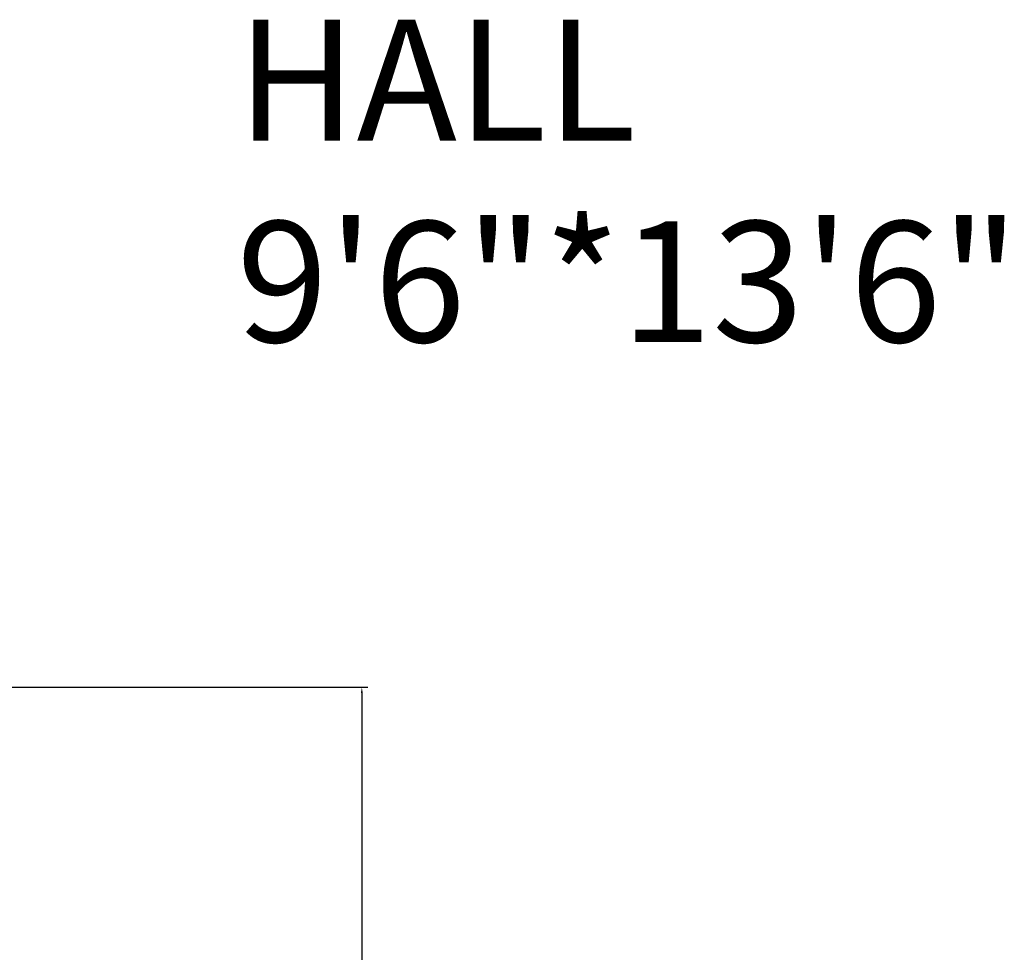
# Model space of a CAD drawing. Units: inches. Extents: x 1998 to 2588, y 1139 to 1977.
# Tile 55 of 134: x 2257 to 2287, y 1663 to 1692. Entities that reach past the tile are written whole.
import ezdxf

# ---------------------------------------------------------------- set-up
doc = ezdxf.new("R2010")
doc.units = ezdxf.units.IN
doc.layers.add('A-ANNO-DIMS', color=2, linetype='Continuous', lineweight=18)
doc.layers.add('A-AREA-IDEN', color=7, linetype='Continuous', lineweight=18)
doc.styles.get("Standard").update_dxf_attribs({"font": 'arial.ttf'})
doc.dimstyles.get("Standard").update_dxf_attribs({"dimtxt": 0.18, "dimasz": 0.18, "dimexe": 0.18, "dimexo": 0.0625, "dimgap": 0.09, "dimtad": 0, "dimtih": 1, "dimtoh": 1, "dimdec": 4, "dimzin": 0, "dimdsep": 46, "dimtxsty": 'Standard', "dimcen": 0.09, "dimadec": 0, "dimazin": 0, "dimtfac": 1, "dimtdec": 4, "dimtofl": 0, "dimtmove": 0, "dimatfit": 3, "dimfxl": 1, "dimtolj": 1, "dimtzin": 0, "dimarcsym": 0})

# ---------------------------------------------------------------- blocks, each defined once
blk = doc.blocks.new('*D11')
at = {"layer": 'A-ANNO-DIMS', "color": 0, "lineweight": -2, "transparency": 16777216}
for p, q in [((2256.378, 1671.356), (2267.646, 1671.356)), ((2267.466, 1671.176), (2267.466, 1634.372)), ((2267.466, 1597.201), (2267.466, 1634.005)), ((2256.378, 1597.021), (2267.646, 1597.021))]:
    blk.add_line(p, q, dxfattribs=at)
at = {"layer": 'A-ANNO-DIMS', "color": 0, "transparency": 16777216}
for points in [[(2267.436, 1671.176), (2267.496, 1671.176), (2267.466, 1671.356)], [(2267.436, 1597.201), (2267.496, 1597.201), (2267.466, 1597.021)]]:
    blk.add_solid(points, dxfattribs=at)
at = {"layer": 'Defpoints', "color": 0, "transparency": 16777216}
for p in [(2256.316, 1671.356), (2256.316, 1597.021), (2267.466, 1597.021)]:
    blk.add_point(p, dxfattribs=at)
at = {"layer": 'A-ANNO-DIMS', "color": 0, "transparency": 16777216, "insert": (2267.466, 1634.189), "char_height": 0.18, "attachment_point": 5}
blk.add_mtext('\\A1;SOFA 74 TYP.', dxfattribs=at)

msp = doc.modelspace()

# ---------------------------------------------------------------- texts
at = {"layer": 'A-AREA-IDEN', "insert": (2263.6329, 1691.7777), "char_height": 3.69875, "attachment_point": 1}
msp.add_mtext_dynamic_manual_height_columns('HALL\\P9\'6"*13\'6"', width=110.572713, gutter_width=18.4938, heights=[0], dxfattribs=at)

# ---------------------------------------------------------------- dimensions: what is measured, and where the dimension line sits
at = {"layer": 'A-ANNO-DIMS'}
dim = msp.add_linear_dim(base=(2267.4662, 1597.0205), p1=(2256.3158, 1671.3565), p2=(2256.3158, 1597.0205), angle=270, text='SOFA <> TYP.', dimstyle='Standard', override={"dimdec": 0, "dimlfac": 1, "dimrnd": 0, "dimzin": 0, "dimdsep": 46, "dimlunit": 2}, dxfattribs=at)
dim.commit()
dim.dimension.update_dxf_attribs({"geometry": '*D11', "text_midpoint": (2267.4662, 1634.1885)})

doc.saveas('drawing.dxf')
